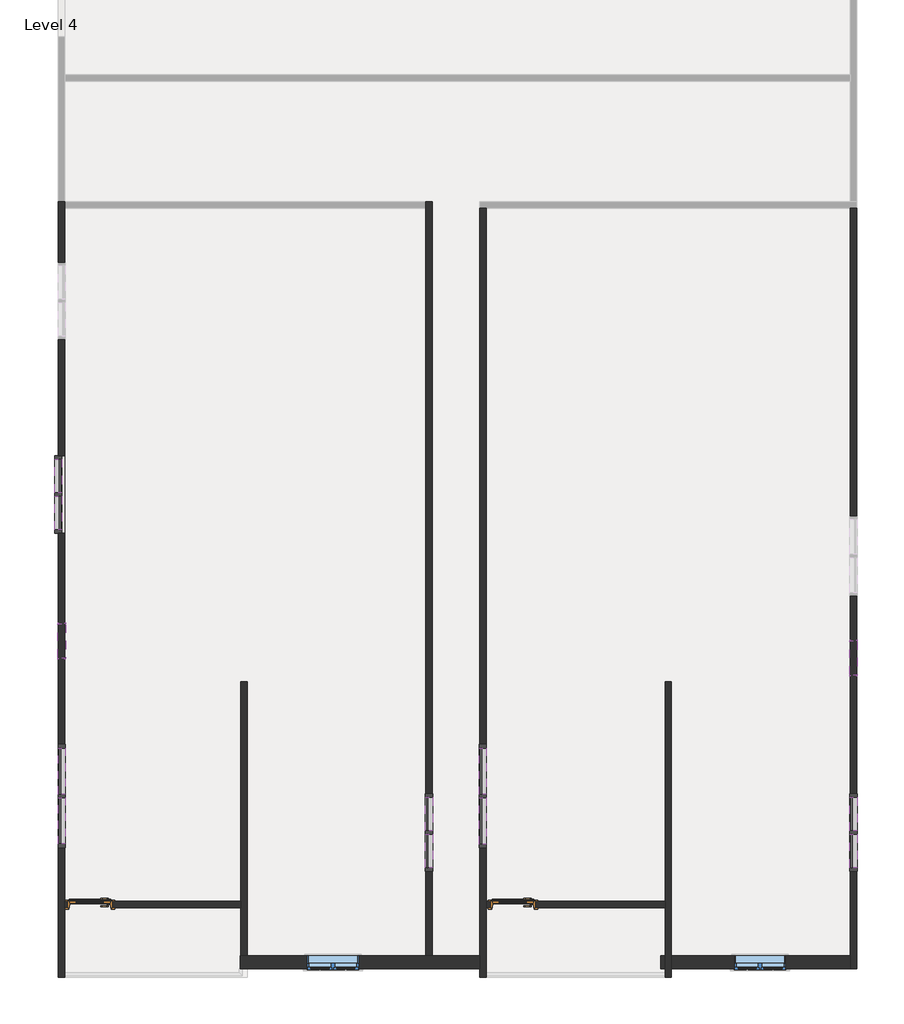
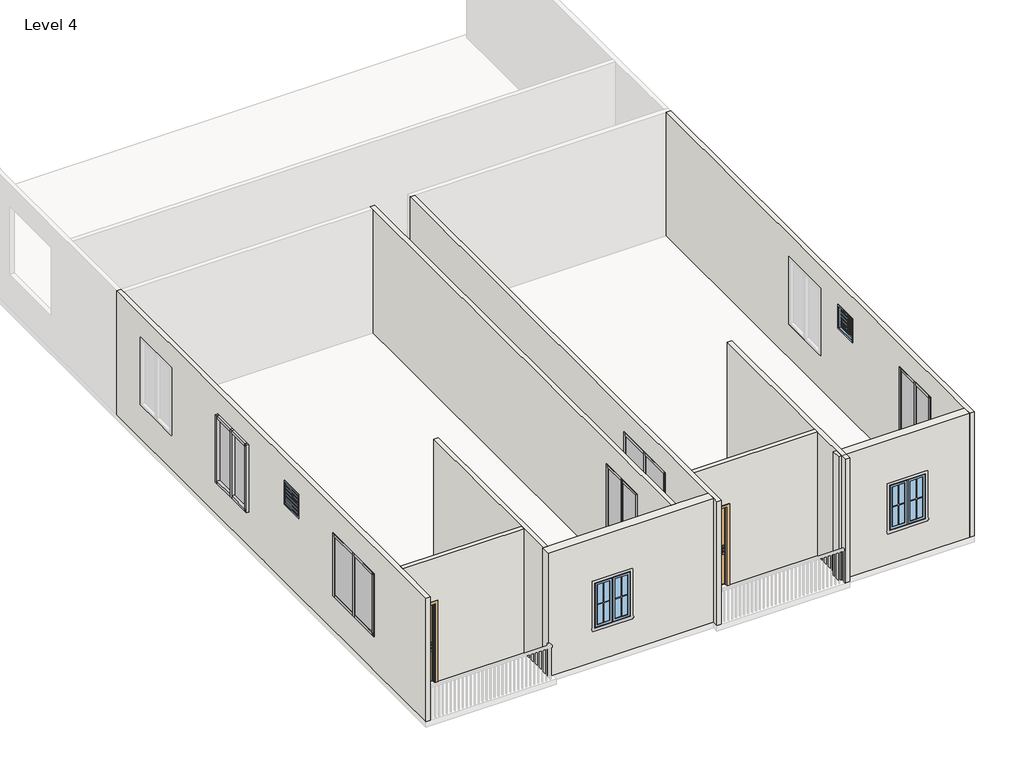
# One storey, part 1 of 3: 35 members, 10 plates, 10 walls, 4 windows, 2 doors.
"""IFC4 building model written with IfcOpenShell, lengths in millimetres."""

from ifc_helpers import new_model, si_unit, frame, origin, place, context, project, spatial, polyline, outline, extrude, faceted_brep, transform, mapped, element, save
from components import door_b81be692, member_8acf8d94, member_501b078b, member_2e6d4a6b, member_96ae0c19, member_d60e8053, member_2fae0574, member_b8ac15de, member_17644e48, system_panel_glazed_c4393626, system_panel_glazed_0e71bc1b, system_panel_glazed_e97abd02, system_panel_glazed_a7ecbca6, window_d341e8ac, window_d39e7ecb

model = new_model("IFC4")

# Units and contexts
model_context = context("Model", 3, world=origin())
ifc_project = project(units=[si_unit("LENGTHUNIT", "METRE", prefix="MILLI")], contexts=[model_context])

# Site, building, storey
site = spatial("IfcSite", under=ifc_project)
building = spatial("IfcBuilding", under=site)
storey = spatial("IfcBuildingStorey", under=building, Name="Level 4", Elevation=10058.4)

# Doors
placement = place(None, origin())
door_shape = door_b81be692(model_context)
element("IfcDoor", 1, ObjectType="29\" x 84\"", at=placement, inside=storey, context=model_context, shape_type="MappedRepresentation", body=[
    mapped(door_shape, transform((-7651.507583, -9448.7163489, 10058.4), x_axis=(1.0, 0.0, 0.0), y_axis=(0.0, 1.0, 0.0), z_axis=(0.0, 0.0, 1.0))),
])
element("IfcDoor", 2, ObjectType="29\" x 84\"", at=placement, inside=storey, context=model_context, shape_type="MappedRepresentation", body=[
    mapped(door_shape, transform((-172.2931282, -9448.9038009, 10058.4), x_axis=(1.0, 0.0, 0.0), y_axis=(0.0, 1.0, 0.0), z_axis=(0.0, 0.0, 1.0))),
])

# Members
member_shape = member_8acf8d94(model_context)
element("IfcMember", 3, ObjectType="Rectangular Mullion : 2.5\" x 5\" rectangular", at=placement, inside=storey, context=model_context, shape_type="MappedRepresentation", body=[
    mapped(member_shape, transform((-8153.157583, -8377.1401329, 12680.286558), x_axis=(0.0, 0.0, 1.0), y_axis=(-1.0, 0.0, 0.0), z_axis=(0.0, -1.0, 0.0))),
])
element("IfcMember", 4, ObjectType="Rectangular Mullion : 2.5\" x 5\" rectangular", at=placement, inside=storey, context=model_context, shape_type="MappedRepresentation", body=[
    mapped(member_shape, transform((-8153.157583, -7497.6651329, 12680.286558), x_axis=(0.0, 0.0, 1.0), y_axis=(-1.0, 0.0, 0.0), z_axis=(0.0, -1.0, 0.0))),
])
element("IfcMember", 5, ObjectType="Rectangular Mullion : 2.5\" x 5\" rectangular", at=placement, inside=storey, context=model_context, shape_type="MappedRepresentation", body=[
    mapped(member_shape, transform((-8153.157583, -6681.6901329, 10972.8), x_axis=(0.0, 0.0, -1.0), y_axis=(-1.0, 0.0, 0.0), z_axis=(0.0, 1.0, 0.0))),
])
element("IfcMember", 6, ObjectType="Rectangular Mullion : 2.5\" x 5\" rectangular", at=placement, inside=storey, context=model_context, shape_type="MappedRepresentation", body=[
    mapped(member_shape, transform((-8153.157583, -7561.1651329, 10972.8), x_axis=(0.0, 0.0, -1.0), y_axis=(-1.0, 0.0, 0.0), z_axis=(0.0, 1.0, 0.0))),
])
member_2_shape = member_501b078b(model_context)
element("IfcMember", 7, ObjectType="Rectangular Mullion : 2.5\" x 5\" rectangular", at=placement, inside=storey, context=model_context, shape_type="MappedRepresentation", body=[
    mapped(member_2_shape, transform((5848.1708786, -8795.0998253, 12801.6), x_axis=(0.0, 0.0, 1.0), y_axis=(-1.0, 0.0, 0.0), z_axis=(0.0, -1.0, 0.0))),
])
element("IfcMember", 8, ObjectType="Rectangular Mullion : 2.5\" x 5\" rectangular", at=placement, inside=storey, context=model_context, shape_type="MappedRepresentation", body=[
    mapped(member_2_shape, transform((5848.1708786, -8142.1745373, 12801.6), x_axis=(0.0, 0.0, 1.0), y_axis=(-1.0, 0.0, 0.0), z_axis=(0.0, -1.0, 0.0))),
])
element("IfcMember", 9, ObjectType="Rectangular Mullion : 2.5\" x 5\" rectangular", at=placement, inside=storey, context=model_context, shape_type="MappedRepresentation", body=[
    mapped(member_2_shape, transform((-1656.4435762, -8795.0998253, 12801.6), x_axis=(0.0, 0.0, 1.0), y_axis=(-1.0, 0.0, 0.0), z_axis=(0.0, -1.0, 0.0))),
])
element("IfcMember", 10, ObjectType="Rectangular Mullion : 2.5\" x 5\" rectangular", at=placement, inside=storey, context=model_context, shape_type="MappedRepresentation", body=[
    mapped(member_2_shape, transform((-1656.4435762, -8142.1745373, 12801.6), x_axis=(0.0, 0.0, 1.0), y_axis=(-1.0, 0.0, 0.0), z_axis=(0.0, -1.0, 0.0))),
])
element("IfcMember", 11, ObjectType="Rectangular Mullion : 2.5\" x 5\" rectangular", at=placement, inside=storey, context=model_context, shape_type="MappedRepresentation", body=[
    mapped(member_2_shape, transform((5848.1708786, -7552.7492493, 10972.8), x_axis=(0.0, 0.0, -1.0), y_axis=(-1.0, 0.0, 0.0), z_axis=(0.0, 1.0, 0.0))),
])
element("IfcMember", 12, ObjectType="Rectangular Mullion : 2.5\" x 5\" rectangular", at=placement, inside=storey, context=model_context, shape_type="MappedRepresentation", body=[
    mapped(member_2_shape, transform((5848.1708786, -8205.6745373, 10972.8), x_axis=(0.0, 0.0, -1.0), y_axis=(-1.0, 0.0, 0.0), z_axis=(0.0, 1.0, 0.0))),
])
element("IfcMember", 13, ObjectType="Rectangular Mullion : 2.5\" x 5\" rectangular", at=placement, inside=storey, context=model_context, shape_type="MappedRepresentation", body=[
    mapped(member_2_shape, transform((-1656.4435762, -7552.7492493, 10972.8), x_axis=(0.0, 0.0, -1.0), y_axis=(-1.0, 0.0, 0.0), z_axis=(0.0, 1.0, 0.0))),
])
element("IfcMember", 14, ObjectType="Rectangular Mullion : 2.5\" x 5\" rectangular", at=placement, inside=storey, context=model_context, shape_type="MappedRepresentation", body=[
    mapped(member_2_shape, transform((-1656.4435762, -8205.6745373, 10972.8), x_axis=(0.0, 0.0, -1.0), y_axis=(-1.0, 0.0, 0.0), z_axis=(0.0, 1.0, 0.0))),
])
member_3_shape = member_2e6d4a6b(model_context)
element("IfcMember", 15, ObjectType="Rectangular Mullion : 2.5\" x 5\" rectangular", at=placement, inside=storey, context=model_context, shape_type="MappedRepresentation", body=[
    mapped(member_3_shape, transform((-705.6931282, -8380.4909009, 12801.6), x_axis=(0.0, 0.0, 1.0), y_axis=(-1.0, 0.0, 0.0), z_axis=(0.0, -1.0, 0.0))),
])
element("IfcMember", 16, ObjectType="Rectangular Mullion : 2.5\" x 5\" rectangular", at=placement, inside=storey, context=model_context, shape_type="MappedRepresentation", body=[
    mapped(member_3_shape, transform((-705.6931282, -7499.3405169, 12801.6), x_axis=(0.0, 0.0, 1.0), y_axis=(-1.0, 0.0, 0.0), z_axis=(0.0, -1.0, 0.0))),
])
element("IfcMember", 17, ObjectType="Rectangular Mullion : 2.5\" x 5\" rectangular", at=placement, inside=storey, context=model_context, shape_type="MappedRepresentation", body=[
    mapped(member_3_shape, transform((-705.6931282, -6681.6901329, 10972.8), x_axis=(0.0, 0.0, -1.0), y_axis=(-1.0, 0.0, 0.0), z_axis=(0.0, 1.0, 0.0))),
])
element("IfcMember", 18, ObjectType="Rectangular Mullion : 2.5\" x 5\" rectangular", at=placement, inside=storey, context=model_context, shape_type="MappedRepresentation", body=[
    mapped(member_3_shape, transform((-705.6931282, -7562.8405169, 10972.8), x_axis=(0.0, 0.0, -1.0), y_axis=(-1.0, 0.0, 0.0), z_axis=(0.0, 1.0, 0.0))),
])
member_4_shape = member_96ae0c19(model_context)
element("IfcMember", 19, ObjectType="Rectangular Mullion : 2.5\" x 5\" rectangular", at=placement, inside=storey, context=model_context, shape_type="MappedRepresentation", body=[
    mapped(member_4_shape, transform((-8210.307583, -2819.4060617, 12801.6), x_axis=(0.0, 0.0, 1.0), y_axis=(-1.0, 0.0, 0.0), z_axis=(0.0, -1.0, 0.0))),
])
element("IfcMember", 20, ObjectType="Rectangular Mullion : 2.5\" x 5\" rectangular", at=placement, inside=storey, context=model_context, shape_type="MappedRepresentation", body=[
    mapped(member_4_shape, transform((-8210.307583, -2164.5788979, 12801.6), x_axis=(0.0, 0.0, 1.0), y_axis=(-1.0, 0.0, 0.0), z_axis=(0.0, -1.0, 0.0))),
])
element("IfcMember", 21, ObjectType="Rectangular Mullion : 2.5\" x 5\" rectangular", at=placement, inside=storey, context=model_context, shape_type="MappedRepresentation", body=[
    mapped(member_4_shape, transform((-8210.307583, -1573.2517341, 10972.8), x_axis=(0.0, 0.0, -1.0), y_axis=(-1.0, 0.0, 0.0), z_axis=(0.0, 1.0, 0.0))),
])
element("IfcMember", 22, ObjectType="Rectangular Mullion : 2.5\" x 5\" rectangular", at=placement, inside=storey, context=model_context, shape_type="MappedRepresentation", body=[
    mapped(member_4_shape, transform((-8210.307583, -2228.0788979, 10972.8), x_axis=(0.0, 0.0, -1.0), y_axis=(-1.0, 0.0, 0.0), z_axis=(0.0, 1.0, 0.0))),
])
member_5_shape = member_d60e8053(model_context)
element("IfcMember", 23, ObjectType="Rectangular Mullion : 2.5\" x 5\" rectangular", at=placement, inside=storey, context=model_context, shape_type="MappedRepresentation", body=[
    mapped(member_5_shape, transform((-8210.307583, -2196.3288979, 10972.8), x_axis=(0.0, -1.0, 0.0), y_axis=(-1.0, 0.0, 0.0), z_axis=(0.0, 0.0, -1.0))),
])
member_6_shape = member_2fae0574(model_context)
element("IfcMember", 24, ObjectType="Rectangular Mullion : 2.5\" x 5\" rectangular", at=placement, inside=storey, context=model_context, shape_type="MappedRepresentation", body=[
    mapped(member_6_shape, transform((-8210.307583, -1509.7517341, 12801.6), x_axis=(0.0, 1.0, 0.0), y_axis=(-1.0, 0.0, 0.0), z_axis=(0.0, 0.0, 1.0))),
])
element("IfcMember", 25, ObjectType="Rectangular Mullion : 2.5\" x 5\" rectangular", at=placement, inside=storey, context=model_context, shape_type="MappedRepresentation", body=[
    mapped(member_6_shape, transform((-8210.307583, -2882.9060617, 10972.8), x_axis=(0.0, -1.0, 0.0), y_axis=(-1.0, 0.0, 0.0), z_axis=(0.0, 0.0, -1.0))),
])
member_7_shape = member_b8ac15de(model_context)
element("IfcMember", 26, ObjectType="Rectangular Mullion : 2.5\" x 5\" rectangular", at=placement, inside=storey, context=model_context, shape_type="MappedRepresentation", body=[
    mapped(member_7_shape, transform((-8153.157583, -7529.4151329, 10972.8), x_axis=(0.0, -1.0, 0.0), y_axis=(-1.0, 0.0, 0.0), z_axis=(0.0, 0.0, -1.0))),
])
member_8_shape = member_17644e48(model_context)
element("IfcMember", 27, ObjectType="Rectangular Mullion : 2.5\" x 5\" rectangular", at=placement, inside=storey, context=model_context, shape_type="MappedRepresentation", body=[
    mapped(member_8_shape, transform((-8153.157583, -6618.1901329, 12680.286558), x_axis=(0.0, 1.0, 0.0), y_axis=(-1.0, 0.0, 0.0), z_axis=(0.0, 0.0, 1.0))),
])
element("IfcMember", 28, ObjectType="Rectangular Mullion : 2.5\" x 5\" rectangular", at=placement, inside=storey, context=model_context, shape_type="MappedRepresentation", body=[
    mapped(member_8_shape, transform((-8153.157583, -8440.6401329, 10972.8), x_axis=(0.0, -1.0, 0.0), y_axis=(-1.0, 0.0, 0.0), z_axis=(0.0, 0.0, -1.0))),
])
element("IfcMember", 29, ObjectType="Rectangular Mullion : 2.5\" x 5\" rectangular", at=placement, inside=storey, context=model_context, shape_type="MappedRepresentation", body=[
    mapped(member_5_shape, transform((5848.1708786, -8173.9245373, 10972.8), x_axis=(0.0, -1.0, 0.0), y_axis=(-1.0, 0.0, 0.0), z_axis=(0.0, 0.0, -1.0))),
])
element("IfcMember", 30, ObjectType="Rectangular Mullion : 2.5\" x 5\" rectangular", at=placement, inside=storey, context=model_context, shape_type="MappedRepresentation", body=[
    mapped(member_5_shape, transform((-1656.4435762, -8173.9245373, 10972.8), x_axis=(0.0, -1.0, 0.0), y_axis=(-1.0, 0.0, 0.0), z_axis=(0.0, 0.0, -1.0))),
])
element("IfcMember", 31, ObjectType="Rectangular Mullion : 2.5\" x 5\" rectangular", at=placement, inside=storey, context=model_context, shape_type="MappedRepresentation", body=[
    mapped(member_5_shape, transform((-705.6931282, -7531.0905169, 10972.8), x_axis=(0.0, -1.0, 0.0), y_axis=(-1.0, 0.0, 0.0), z_axis=(0.0, 0.0, -1.0))),
])
element("IfcMember", 32, ObjectType="Rectangular Mullion : 2.5\" x 5\" rectangular", at=placement, inside=storey, context=model_context, shape_type="MappedRepresentation", body=[
    mapped(member_6_shape, transform((5848.1708786, -7489.2492493, 12801.6), x_axis=(0.0, 1.0, 0.0), y_axis=(-1.0, 0.0, 0.0), z_axis=(0.0, 0.0, 1.0))),
])
element("IfcMember", 33, ObjectType="Rectangular Mullion : 2.5\" x 5\" rectangular", at=placement, inside=storey, context=model_context, shape_type="MappedRepresentation", body=[
    mapped(member_6_shape, transform((-1656.4435762, -7489.2492493, 12801.6), x_axis=(0.0, 1.0, 0.0), y_axis=(-1.0, 0.0, 0.0), z_axis=(0.0, 0.0, 1.0))),
])
element("IfcMember", 34, ObjectType="Rectangular Mullion : 2.5\" x 5\" rectangular", at=placement, inside=storey, context=model_context, shape_type="MappedRepresentation", body=[
    mapped(member_6_shape, transform((-705.6931282, -6618.1901329, 12801.6), x_axis=(0.0, 1.0, 0.0), y_axis=(-1.0, 0.0, 0.0), z_axis=(0.0, 0.0, 1.0))),
])
element("IfcMember", 35, ObjectType="Rectangular Mullion : 2.5\" x 5\" rectangular", at=placement, inside=storey, context=model_context, shape_type="MappedRepresentation", body=[
    mapped(member_6_shape, transform((5848.1708786, -8858.5998253, 10972.8), x_axis=(0.0, -1.0, 0.0), y_axis=(-1.0, 0.0, 0.0), z_axis=(0.0, 0.0, -1.0))),
])
element("IfcMember", 36, ObjectType="Rectangular Mullion : 2.5\" x 5\" rectangular", at=placement, inside=storey, context=model_context, shape_type="MappedRepresentation", body=[
    mapped(member_6_shape, transform((-1656.4435762, -8858.5998253, 10972.8), x_axis=(0.0, -1.0, 0.0), y_axis=(-1.0, 0.0, 0.0), z_axis=(0.0, 0.0, -1.0))),
])
element("IfcMember", 37, ObjectType="Rectangular Mullion : 2.5\" x 5\" rectangular", at=placement, inside=storey, context=model_context, shape_type="MappedRepresentation", body=[
    mapped(member_6_shape, transform((-705.6931282, -8443.9909009, 10972.8), x_axis=(0.0, -1.0, 0.0), y_axis=(-1.0, 0.0, 0.0), z_axis=(0.0, 0.0, -1.0))),
])

# Plates
system_panel_glazed_shape = system_panel_glazed_c4393626(model_context)
element("IfcPlate", 38, ObjectType="System Panel : Glazed", at=placement, inside=storey, context=model_context, shape_type="MappedRepresentation", body=[
    mapped(system_panel_glazed_shape, transform((-8210.307583, -1868.915316, 11036.3), x_axis=(0.0, -1.0, 0.0), y_axis=(1.0, 0.0, 0.0), z_axis=(0.0, 0.0, 1.0))),
])
element("IfcPlate", 39, ObjectType="System Panel : Glazed", at=placement, inside=storey, context=model_context, shape_type="MappedRepresentation", body=[
    mapped(system_panel_glazed_shape, transform((-8210.307583, -2523.7424798, 11036.3), x_axis=(0.0, -1.0, 0.0), y_axis=(1.0, 0.0, 0.0), z_axis=(0.0, 0.0, 1.0))),
])
system_panel_glazed_2_shape = system_panel_glazed_0e71bc1b(model_context)
element("IfcPlate", 40, ObjectType="System Panel : Glazed", at=placement, inside=storey, context=model_context, shape_type="MappedRepresentation", body=[
    mapped(system_panel_glazed_2_shape, transform((-8153.157583, -7089.6776329, 11036.3), x_axis=(0.0, -1.0, 0.0), y_axis=(1.0, 0.0, 0.0), z_axis=(0.0, 0.0, 1.0))),
])
element("IfcPlate", 41, ObjectType="System Panel : Glazed", at=placement, inside=storey, context=model_context, shape_type="MappedRepresentation", body=[
    mapped(system_panel_glazed_2_shape, transform((-8153.157583, -7969.1526329, 11036.3), x_axis=(0.0, -1.0, 0.0), y_axis=(1.0, 0.0, 0.0), z_axis=(0.0, 0.0, 1.0))),
])
system_panel_glazed_3_shape = system_panel_glazed_e97abd02(model_context)
element("IfcPlate", 42, ObjectType="System Panel : Glazed", at=placement, inside=storey, context=model_context, shape_type="MappedRepresentation", body=[
    mapped(system_panel_glazed_3_shape, transform((5848.1708786, -7847.4618933, 11036.3), x_axis=(0.0, -1.0, 0.0), y_axis=(1.0, 0.0, 0.0), z_axis=(0.0, 0.0, 1.0))),
])
element("IfcPlate", 43, ObjectType="System Panel : Glazed", at=placement, inside=storey, context=model_context, shape_type="MappedRepresentation", body=[
    mapped(system_panel_glazed_3_shape, transform((-1656.4435762, -7847.4618933, 11036.3), x_axis=(0.0, -1.0, 0.0), y_axis=(1.0, 0.0, 0.0), z_axis=(0.0, 0.0, 1.0))),
])
element("IfcPlate", 44, ObjectType="System Panel : Glazed", at=placement, inside=storey, context=model_context, shape_type="MappedRepresentation", body=[
    mapped(system_panel_glazed_3_shape, transform((5848.1708786, -8500.3871813, 11036.3), x_axis=(0.0, -1.0, 0.0), y_axis=(1.0, 0.0, 0.0), z_axis=(0.0, 0.0, 1.0))),
])
element("IfcPlate", 45, ObjectType="System Panel : Glazed", at=placement, inside=storey, context=model_context, shape_type="MappedRepresentation", body=[
    mapped(system_panel_glazed_3_shape, transform((-1656.4435762, -8500.3871813, 11036.3), x_axis=(0.0, -1.0, 0.0), y_axis=(1.0, 0.0, 0.0), z_axis=(0.0, 0.0, 1.0))),
])
system_panel_glazed_4_shape = system_panel_glazed_a7ecbca6(model_context)
element("IfcPlate", 46, ObjectType="System Panel : Glazed", at=placement, inside=storey, context=model_context, shape_type="MappedRepresentation", body=[
    mapped(system_panel_glazed_4_shape, transform((-705.6931282, -7090.5153249, 11036.3), x_axis=(0.0, -1.0, 0.0), y_axis=(1.0, 0.0, 0.0), z_axis=(0.0, 0.0, 1.0))),
])
element("IfcPlate", 47, ObjectType="System Panel : Glazed", at=placement, inside=storey, context=model_context, shape_type="MappedRepresentation", body=[
    mapped(system_panel_glazed_4_shape, transform((-705.6931282, -7971.6657089, 11036.3), x_axis=(0.0, -1.0, 0.0), y_axis=(1.0, 0.0, 0.0), z_axis=(0.0, 0.0, 1.0))),
])

# Walls
element("IfcWall", 48, ObjectType="4.5\" wall", at=placement, inside=storey, context=model_context, shape_type="Brep", body=[
    faceted_brep([(-8096.007583, -10738.0280197, 10058.4), (-8096.007583, -9509.0413489, 10058.4), (-8096.007583, -9394.7413489, 10058.4), (-8096.007583, 2864.0002499, 10058.4), (-8096.007583, 2978.3002499, 10058.4), (-8096.007583, 2978.3002499, 13411.2), (-8096.007583, 2864.0002499, 13411.2), (-8096.007583, -9394.7413489, 13411.2), (-8096.007583, -9509.0413489, 13411.2), (-8096.007583, -10738.0280197, 13411.2), (-8096.007583, -6618.1901329, 12680.286558), (-8096.007583, -6618.1901329, 10972.8), (-8096.007583, -8440.6401329, 10972.8), (-8096.007583, -8440.6401329, 12680.286558), (-8096.007583, -5094.1901329, 12172.95), (-8096.007583, -5094.1901329, 12782.55), (-8096.007583, -4484.5901329, 12782.55), (-8096.007583, -4484.5901329, 12172.95), (-8096.007583, 1909.8209543, 12801.6), (-8096.007583, 1909.8209543, 10972.8), (-8096.007583, 536.6666267, 10972.8), (-8096.007583, 536.6666267, 12801.6), (-8096.007583, -1509.7517341, 12801.6), (-8096.007583, -1509.7517341, 10972.8), (-8096.007583, -2882.9060617, 10972.8), (-8096.007583, -2882.9060617, 12801.6), (-8210.307583, 2978.3002499, 10058.4), (-8210.307583, -10738.0280197, 10058.4), (-8210.307583, -10738.0280197, 13411.2), (-8210.307583, 2978.3002499, 13411.2), (-8210.307583, -6618.1901329, 10972.8), (-8210.307583, -6618.1901329, 12680.286558), (-8210.307583, -8440.6401329, 12680.286558), (-8210.307583, -8440.6401329, 10972.8), (-8210.307583, -5094.1901329, 12782.55), (-8210.307583, -5094.1901329, 12172.95), (-8210.307583, -4484.5901329, 12172.95), (-8210.307583, -4484.5901329, 12782.55), (-8210.307583, 1909.8209543, 10972.8), (-8210.307583, 1909.8209543, 12801.6), (-8210.307583, 536.6666267, 12801.6), (-8210.307583, 536.6666267, 10972.8), (-8210.307583, -1509.7517341, 10972.8), (-8210.307583, -1509.7517341, 12801.6), (-8210.307583, -2882.9060617, 12801.6), (-8210.307583, -2882.9060617, 10972.8)], [[[0, 1, 2, 3, 4, 5, 6, 7, 8, 9], [10, 11, 12, 13], [14, 15, 16, 17], [18, 19, 20, 21], [22, 23, 24, 25]], [[26, 27, 28, 29], [30, 31, 32, 33], [34, 35, 36, 37], [38, 39, 40, 41], [42, 43, 44, 45]], [[4, 3, 2, 1, 0, 27, 26]], [[9, 8, 7, 6, 5, 29, 28]], [[0, 9, 28, 27]], [[5, 4, 26, 29]], [[10, 31, 30, 11]], [[31, 10, 13, 32]], [[32, 13, 12, 33]], [[11, 30, 33, 12]], [[35, 34, 15, 14]], [[36, 35, 14, 17]], [[37, 36, 17, 16]], [[34, 37, 16, 15]], [[38, 19, 18, 39]], [[39, 18, 21, 40]], [[40, 21, 20, 41]], [[19, 38, 41, 20]], [[22, 43, 42, 23]], [[43, 22, 25, 44]], [[44, 25, 24, 45]], [[23, 42, 45, 24]]]),
])
element("IfcWall", 49, ObjectType="4.5\" wall", at=placement, inside=storey, context=model_context, shape_type="Brep", body=[
    faceted_brep([(-1599.2935762, -10357.2779557, 10058.4), (-1599.2935762, 2978.3002499, 10058.4), (-1599.2935762, 2978.3002499, 13411.2), (-1599.2935762, -10357.2779557, 13411.2), (-1599.2935762, -7489.2492493, 12801.6), (-1599.2935762, -7489.2492493, 10972.8), (-1599.2935762, -8858.5998253, 10972.8), (-1599.2935762, -8858.5998253, 12801.6), (-1713.5935762, 2978.3002499, 10058.4), (-1713.5935762, 2864.0002499, 10058.4), (-1713.5935762, -10357.2779557, 10058.4), (-1713.5935762, -10357.2779557, 13411.2), (-1713.5935762, 2864.0002499, 13411.2), (-1713.5935762, 2978.3002499, 13411.2), (-1713.5935762, -7489.2492493, 10972.8), (-1713.5935762, -7489.2492493, 12801.6), (-1713.5935762, -8858.5998253, 12801.6), (-1713.5935762, -8858.5998253, 10972.8)], [[[0, 1, 2, 3], [4, 5, 6, 7]], [[8, 9, 10, 11, 12, 13], [14, 15, 16, 17]], [[1, 0, 10, 9, 8]], [[3, 2, 13, 12, 11]], [[2, 1, 8, 13]], [[0, 3, 11, 10]], [[14, 5, 4, 15]], [[15, 4, 7, 16]], [[16, 7, 6, 17]], [[5, 14, 17, 6]]]),
])
element("IfcWall", 50, ObjectType="4.5\" wall", at=placement, inside=storey, context=model_context, shape_type="Brep", body=[
    faceted_brep([(5791.0208786, 2864.0002499, 10058.4), (5791.0208786, -10357.2779557, 10058.4), (5791.0208786, -10585.8779557, 10058.4), (5791.0208786, -10585.8779557, 13411.2), (5791.0208786, -10357.2779557, 13411.2), (5791.0208786, 2864.0002499, 13411.2), (5791.0208786, -7489.2492493, 10972.8), (5791.0208786, -7489.2492493, 12801.6), (5791.0208786, -8858.5998253, 12801.6), (5791.0208786, -8858.5998253, 10972.8), (5791.0208786, -2574.8021821, 10972.8), (5791.0208786, -2574.8021821, 12801.6), (5791.0208786, -3997.2021821, 12801.6), (5791.0208786, -3997.2021821, 10972.8), (5791.0208786, -4784.6021821, 12211.05), (5791.0208786, -4784.6021821, 12820.65), (5791.0208786, -5394.2021821, 12820.65), (5791.0208786, -5394.2021821, 12211.05), (5905.3208786, -10585.8779557, 10058.4), (5905.3208786, 2864.0002499, 10058.4), (5905.3208786, 2864.0002499, 13411.2), (5905.3208786, -10585.8779557, 13411.2), (5905.3208786, -7489.2492493, 12801.6), (5905.3208786, -7489.2492493, 10972.8), (5905.3208786, -8858.5998253, 10972.8), (5905.3208786, -8858.5998253, 12801.6), (5905.3208786, -2574.8021821, 12801.6), (5905.3208786, -2574.8021821, 10972.8), (5905.3208786, -3997.2021821, 10972.8), (5905.3208786, -3997.2021821, 12801.6), (5905.3208786, -4784.6021821, 12820.65), (5905.3208786, -4784.6021821, 12211.05), (5905.3208786, -5394.2021821, 12211.05), (5905.3208786, -5394.2021821, 12820.65)], [[[0, 1, 2, 3, 4, 5], [6, 7, 8, 9], [10, 11, 12, 13], [14, 15, 16, 17]], [[18, 19, 20, 21], [22, 23, 24, 25], [26, 27, 28, 29], [30, 31, 32, 33]], [[2, 1, 0, 19, 18]], [[5, 4, 3, 21, 20]], [[0, 5, 20, 19]], [[3, 2, 18, 21]], [[22, 7, 6, 23]], [[7, 22, 25, 8]], [[8, 25, 24, 9]], [[23, 6, 9, 24]], [[10, 27, 26, 11]], [[11, 26, 29, 12]], [[12, 29, 28, 13]], [[27, 10, 13, 28]], [[31, 30, 15, 14]], [[32, 31, 14, 17]], [[33, 32, 17, 16]], [[30, 33, 16, 15]]]),
])
element("IfcWall", 51, ObjectType="4.5\" wall", at=placement, inside=storey, context=model_context, shape_type="Brep", body=[
    faceted_brep([(-762.8431282, 2864.0002499, 10058.4), (-762.8431282, -10357.2779557, 10058.4), (-762.8431282, -10585.8779557, 10058.4), (-762.8431282, -10737.6531157, 10058.4), (-762.8431282, -10737.6531157, 13411.2), (-762.8431282, -10585.8779557, 13411.2), (-762.8431282, -10357.2779557, 13411.2), (-762.8431282, 2864.0002499, 13411.2), (-762.8431282, -6618.1901329, 10972.8), (-762.8431282, -6618.1901329, 12801.6), (-762.8431282, -8443.9909009, 12801.6), (-762.8431282, -8443.9909009, 10972.8), (-648.5431282, -10737.6531157, 10058.4), (-648.5431282, -9509.2288009, 10058.4), (-648.5431282, -9394.9288009, 10058.4), (-648.5431282, 2864.0002499, 10058.4), (-648.5431282, 2864.0002499, 13411.2), (-648.5431282, -9394.9288009, 13411.2), (-648.5431282, -9509.2288009, 13411.2), (-648.5431282, -10737.6531157, 13411.2), (-648.5431282, -6618.1901329, 12801.6), (-648.5431282, -6618.1901329, 10972.8), (-648.5431282, -8443.9909009, 10972.8), (-648.5431282, -8443.9909009, 12801.6)], [[[0, 1, 2, 3, 4, 5, 6, 7], [8, 9, 10, 11]], [[12, 13, 14, 15, 16, 17, 18, 19], [20, 21, 22, 23]], [[3, 2, 1, 0, 15, 14, 13, 12]], [[4, 3, 12, 19]], [[7, 6, 5, 4, 19, 18, 17, 16]], [[8, 21, 20, 9]], [[9, 20, 23, 10]], [[10, 23, 22, 11]], [[21, 8, 11, 22]], [[0, 7, 16, 15]]]),
])
element("IfcWall", 52, ObjectType="4.5\" wall", at=placement, inside=storey, context=model_context, shape_type="Brep", body=[
    faceted_brep([(-4874.3237038, -10357.2779557, 10058.4), (-4874.3237038, -5507.4946657, 10058.4), (-4874.3237038, -5507.4946657, 13411.2), (-4874.3237038, -10357.2779557, 13411.2), (-4988.6237038, -10357.2779557, 10058.4), (-4988.6237038, -10357.2779557, 13411.2), (-4988.6237038, -9509.0413489, 13411.2), (-4988.6237038, -9394.7413489, 13411.2), (-4988.6237038, -5507.4946657, 13411.2), (-4988.6237038, -5507.4946657, 10058.4), (-4988.6237038, -9394.7413489, 10058.4), (-4988.6237038, -9509.0413489, 10058.4)], [[[0, 1, 2, 3]], [[4, 5, 6, 7, 8, 9, 10, 11]], [[1, 0, 4, 11, 10, 9]], [[2, 1, 9, 8]], [[3, 2, 8, 7, 6, 5]], [[0, 3, 5, 4]]]),
])
element("IfcWall", 53, ObjectType="4.5\" wall", at=placement, inside=storey, context=model_context, shape_type="Brep", body=[
    faceted_brep([(2515.990751, -5507.4946657, 10058.4), (2515.990751, -9394.9288009, 10058.4), (2515.990751, -9509.2288009, 10058.4), (2515.990751, -10737.6531157, 10058.4), (2515.990751, -10737.6531157, 13411.2), (2515.990751, -9509.2288009, 13411.2), (2515.990751, -9394.9288009, 13411.2), (2515.990751, -5507.4946657, 13411.2), (2630.290751, -5507.4946657, 10058.4), (2630.290751, -5507.4946657, 13411.2), (2630.290751, -10737.6531157, 13411.2), (2630.290751, -10737.6531157, 10058.4)], [[[0, 1, 2, 3, 4, 5, 6, 7]], [[8, 9, 10, 11]], [[3, 2, 1, 0, 8, 11]], [[4, 3, 11, 10]], [[7, 6, 5, 4, 10, 9]], [[0, 7, 9, 8]]]),
])
element("IfcWall", 54, ObjectType="4.5\" wall", at=placement, inside=storey, context=model_context, shape_type="SweptSolid", body=[
    extrude(outline(polyline([(13411.2, -4988.6237038), (13411.2, -8096.007583), (10058.4, -8096.007583), (10058.4, -8045.207583), (12217.4, -8045.207583), (12217.4, -7257.807583), (10058.4, -7257.807583), (10058.4, -4988.6237038), (13411.2, -4988.6237038)])), frame((0.0, -9509.0413489, 0.0), z_axis=(0.0, 1.0, 0.0), x_axis=(0.0, 0.0, 1.0)), (0.0, 0.0, 1.0), 114.3),
])
element("IfcWall", 55, ObjectType="4.5\" wall", at=placement, inside=storey, context=model_context, shape_type="SweptSolid", body=[
    extrude(outline(polyline([(13411.2, 2515.990751), (13411.2, -648.5431282), (10058.4, -648.5431282), (10058.4, -565.9931282), (12217.4, -565.9931282), (12217.4, 221.4068718), (10058.4, 221.4068718), (10058.4, 2515.990751), (13411.2, 2515.990751)])), frame((0.0, -9509.2288009, 0.0), z_axis=(0.0, 1.0, 0.0), x_axis=(0.0, 0.0, 1.0)), (0.0, 0.0, 1.0), 114.3),
])
element("IfcWall", 56, ObjectType="9\" wall", at=placement, inside=storey, context=model_context, shape_type="Brep", body=[
    faceted_brep([(-762.8431282, -10357.2779557, 10058.4), (-1599.2935762, -10357.2779557, 10058.4), (-1713.5935762, -10357.2779557, 10058.4), (-4874.3237038, -10357.2779557, 10058.4), (-4988.6237038, -10357.2779557, 10058.4), (-4996.231207, -10357.2779557, 10058.4), (-4996.231207, -10357.2779557, 13411.2), (-4988.6237038, -10357.2779557, 13411.2), (-4874.3237038, -10357.2779557, 13411.2), (-1713.5935762, -10357.2779557, 13411.2), (-1599.2935762, -10357.2779557, 13411.2), (-762.8431282, -10357.2779557, 13411.2), (-3813.8737038, -10357.2779557, 12192.0), (-3813.8737038, -10357.2779557, 10972.8), (-2899.4737038, -10357.2779557, 10972.8), (-2899.4737038, -10357.2779557, 12192.0), (-762.8431282, -10585.8779557, 10058.4), (-762.8431282, -10585.8779557, 13411.2), (-4996.231207, -10585.8779557, 13411.2), (-4996.231207, -10585.8779557, 10058.4), (-3813.8737038, -10585.8779557, 12192.0), (-2899.4737038, -10585.8779557, 12192.0), (-2899.4737038, -10585.8779557, 10972.8), (-3813.8737038, -10585.8779557, 10972.8)], [[[0, 1, 2, 3, 4, 5, 6, 7, 8, 9, 10, 11], [12, 13, 14, 15]], [[16, 17, 18, 19], [20, 21, 22, 23]], [[5, 4, 3, 2, 1, 0, 16, 19]], [[6, 5, 19, 18]], [[11, 10, 9, 8, 7, 6, 18, 17]], [[0, 11, 17, 16]], [[13, 12, 20, 23]], [[14, 13, 23, 22]], [[15, 14, 22, 21]], [[12, 15, 21, 20]]]),
])
element("IfcWall", 57, ObjectType="9\" wall", at=placement, inside=storey, context=model_context, shape_type="SweptSolid", body=[
    extrude(outline(polyline([(10058.4, 5791.0208786), (13411.2, 5791.0208786), (13411.2, 2436.2994194), (10058.4, 2436.2994194), (10058.4, 5791.0208786)]), holes=[polyline([(12192.0, 3739.9708786), (12192.0, 4654.3708786), (10972.8, 4654.3708786), (10972.8, 3739.9708786), (12192.0, 3739.9708786)])]), frame((0.0, -10585.8779557, 0.0), z_axis=(0.0, 1.0, 0.0), x_axis=(0.0, 0.0, 1.0)), (0.0, 0.0, 1.0), 228.6),
])

# Windows
window_shape = window_d341e8ac(model_context)
element("IfcWindow", 58, ObjectType="Window-Casement-Double : 36\" x 48\"", at=placement, inside=storey, context=model_context, shape_type="MappedRepresentation", body=[
    mapped(window_shape, transform((-3356.6737038, -10471.5779557, 10058.4), x_axis=(-1.0, 0.0, 0.0), y_axis=(0.0, -1.0, 0.0), z_axis=(0.0, 0.0, 1.0))),
])
element("IfcWindow", 59, ObjectType="Window-Casement-Double : 36\" x 48\"", at=placement, inside=storey, context=model_context, shape_type="MappedRepresentation", body=[
    mapped(window_shape, transform((4197.1708786, -10471.5779557, 10058.4), x_axis=(-1.0, 0.0, 0.0), y_axis=(0.0, -1.0, 0.0), z_axis=(0.0, 0.0, 1.0))),
])
window_2_shape = window_d39e7ecb(model_context)
element("IfcWindow", 60, ObjectType="Window-Louvers : 24\" x 24\"", at=placement, inside=storey, context=model_context, shape_type="MappedRepresentation", body=[
    mapped(window_2_shape, transform((-8159.507583, -4789.3901329, 11258.55), x_axis=(0.0, 1.0, 0.0), y_axis=(-1.0, 0.0, 0.0), z_axis=(0.0, 0.0, 1.0))),
])
element("IfcWindow", 61, ObjectType="Window-Louvers : 24\" x 24\"", at=placement, inside=storey, context=model_context, shape_type="MappedRepresentation", body=[
    mapped(window_2_shape, transform((5854.5208786, -5089.4021821, 11296.65), x_axis=(0.0, -1.0, 0.0), y_axis=(1.0, 0.0, 0.0), z_axis=(0.0, 0.0, 1.0))),
])

save(model, "model.ifc")

# Revit data of these elements
# Type "29\" x 84\""
#   Type Mark = "8"
#   Assembly Code = "B2030100"
#   Analytic Construction = "French door, wood frame with single glass"
#   Threshold Offset [instance default] = 0' - 0 1/2"
#   Thickness = 0' - 1 3/8"
#   Thermal Resistance (R) = 1.0696 (h·ft²·°F)/BTU
#   Swing Angle [instance default] = 90.00°
#   Stiles = 0' - 4 3/4"
#   Rough Width = 2' - 7"
#   Rough Height = 7' - 1"
#   Radius = 1' - 0.00625"
#   Lock Rail = 0' - 7 1/8"
#   Height = 7' - 0"
#   Width = 2' - 5"
#   Heat Transfer Coefficient (U) = 0.9350 BTU/(h·ft²·°F)
#   Door Offset [instance default] = 0' - 0"
#   Bottom Rail = 0' - 9 1/2"
#   Threshold [instance default] = yes
#   Function = 1
#   Exterior Trim [instance default] = yes
#   Trim Material = Cherry
#   Threshold Material = Cherry
#   Panel Material = Cherry
#   Glazing = Glass
#   Frame Material = Cherry
#   Door Handle Material = Aluminum
#   Visual Light Transmittance = 0
#   Solar Heat Gain Coefficient = 0
#   Wall Closure = (empty or 0)
#   Construction Type = (empty or 0)
# Type "Rectangular Mullion : 2.5\" x 5\" rectangular"
#   built-in parameter 1007304 = 0.416667 (stored number, unit not read)
#   built-in parameter 1007301 = 0.104167 (stored number, unit not read)
#   built-in parameter 1007300 = 0.104167 (stored number, unit not read)
# Type "System Panel : Glazed"
#   Construction Type Id = "GSP4R"
#   Analytic Construction = "1/8 in Pilkington single glazing"
#   Visual Light Transmittance = 0.9
#   Solar Heat Gain Coefficient = 0.86
#   Heat Transfer Coefficient (U) = 1.18115 BTU/(h·ft²·°F)
#   Define Thermal Properties by = 1
# Type "4.5\" wall"
#   Assembly Code = "B2010"
#   Layers, outside or top first: 0' - 4 1/2" no material (function 1)
# Type "9\" wall"
#   Assembly Code = "B2010"
#   Layers, outside or top first: 0' - 9" no material (function 1)
# Type "Window-Casement-Double : 36\" x 48\""
#   Type Mark = "14"
#   Fire Rating = "0.5h"
#   Assembly Code = "B2020100"
#   Analytic Construction = "Double glazing - domestic"
#   Frame Extension [instance default] = 0' - 0 1/4"
#   Window Inset [instance default] = 0' - 0"
#   Wall Thickness [instance default] = 0' - 6"
#   Interior Wall Closure [instance default] = 0' - 2 1/4"
#   Half Width = 1' - 6"
#   Visual Light Transmittance = 0.81
#   Thermal Resistance (R) = 1.8146 (h·ft²·°F)/BTU
#   Solar Heat Gain Coefficient = 0.76
#   Rough Width = 3' - 0 1/2"
#   Rough Height = 4' - 0 1/2"
#   Height = 4' - 0"
#   Heat Transfer Coefficient (U) = 0.5511 BTU/(h·ft²·°F)
#   Exterior Wall Closure [instance default] = 0' - 1 1/4"
#   Extension Jamb [instance default] = 0' - 2 1/4"
#   Default Sill Height = 3' - 0"
#   Width = 3' - 0"
#   Define Thermal Properties by = 0
#   Muntin Visibility = yes
#   Interior Trim Visibility [instance default] = yes
#   Exterior Trim Visibility [instance default] = yes
#   Extension Jamb Visibility [instance default] = yes
#   Interior Trim Material = Wood - Stained
#   Muntin Pattern = Muntin Pattern_2x2 : Muntin Pattern_2x2
#   Interior Trim = Trim-Window-Interior-Flat : Picture Frame
#   Interior Frame Material = Wood - Stained
#   Glass Panel Material = Glass
#   Exterior Trim Material = Clad - White
#   Exterior Trim = Trim-Window-Exterior-Flat : with Sill
#   Exterior Frame Material = Clad - White
#   Wall Closure = (empty or 0)
# Type "Window-Louvers : 24\" x 24\""
#   Type Mark = "18"
#   Construction Type Id = "GSP4R"
#   Assembly Code = "B20"
#   Analytic Construction = "1/8 in Pilkington single glazing"
#   Visual Light Transmittance = 0.9
#   Thermal Resistance (R) = 1.53941 (h·ft²·°F)/BTU
#   Solar Heat Gain Coefficient = 0.78
#   Max Height = 1' - 11.74264"
#   Height = 2' - 0"
#   Heat Transfer Coefficient (U) = 0.6496 BTU/(h·ft²·°F)
#   Blade Width [instance default] = 1' - 10 1/2"
#   Blade Vertical Thickness = 0' - 0.35355"
#   Blade Thickness = 0' - 0 1/4"
#   Blade Spacing = 0' - 1 1/2"
#   Blade Height = 0' - 1.85355"
#   Blade Depth = 0' - 3"
#   Blade Angle = 45.00°
#   Default Sill Height = 3' - 0"
#   Trim Projection_Exterior = 0' - 0 1/2"
#   Trim Projection_Interior = 0' - 0 1/2"
#   Trim Width_Exterior = 0' - 1 1/2"
#   Trim Width_Interior = 0' - 1 1/2"
#   Width = 2' - 0"
#   Max Blade Count = 12
#   Define Thermal Properties by = 1
#   Blade Count = 12
#   Frame Material = Birch
#   Louver Material = Birch
#   Trim Exterior Material = Birch
#   Trim Interior Material = Birch
#   Wall Closure = (empty or 0)
# Elements 1, 2 (IfcDoor, "29\" x 84\"")
#   Threshold Offset = 0' - 0 1/2"
#   Swing Angle = 90.00°
#   Door Offset = 0' - 0"
#   Threshold = yes
#   Exterior Trim = yes
#   Phase Created = New Construction
#   Materials on its faces: "Cherry", "Aluminum", "Glass"
# Elements 3, 4, 5, 6, 7, 8, 9, 10, 11, 12, 13, 14, 15, 16, 17, 18, 19, 20, 21, 22, 23, 24, 25, 26, 27, 28, 29, 30, 31, 32, 33, 34, 35, 36, 37 (IfcMember, "Rectangular Mullion : 2.5\" x 5\" rectangular")
#   Phase Created = New Construction
#   Materials on its faces: "Aluminum"
# Elements 38, 39, 40, 41, 42, 43, 44, 45, 46, 47 (IfcPlate, "System Panel : Glazed")
#   Phase Created = New Construction
#   Materials on its faces: "Glass"
# Elements 48, 49, 50, 51, 52, 53, 54, 55 (IfcWall, "4.5\" wall")
#   Top Offset = -1' - 6"
#   Base Offset = 0' - 0"
#   Unconnected Height = 11' - 0"
#   wall height = 11' - 0"
#   Phase Created = New Construction
#   Base Constraint = Level 4
#   Materials on its faces: "Default Wall"
# Elements 56, 57 (IfcWall, "9\" wall")
#   Top Offset = -1' - 6"
#   Base Offset = 0' - 0"
#   Unconnected Height = 11' - 0"
#   wall height = 11' - 0"
#   Phase Created = New Construction
#   Base Constraint = Level 4
#   Materials on its faces: "Default Wall"
# Element 58 (IfcWindow, "Window-Casement-Double : 36\" x 48\"")
#   Mark = "13"
#   Window Inset = 0' - 0"
#   Interior Wall Closure = 0' - 2 1/4"
#   Frame Extension = 0' - 0 1/4"
#   Exterior Wall Closure = 0' - 1 1/4"
#   Interior Trim Visibility = yes
#   Exterior Trim Visibility = yes
#   Phase Created = New Construction
#   Materials on its faces: "Wood - Stained", "Glass", "Clad - White"
# Element 59 (IfcWindow, "Window-Casement-Double : 36\" x 48\"")
#   Mark = "14"
#   Window Inset = 0' - 0"
#   Interior Wall Closure = 0' - 2 1/4"
#   Frame Extension = 0' - 0 1/4"
#   Exterior Wall Closure = 0' - 1 1/4"
#   Interior Trim Visibility = yes
#   Exterior Trim Visibility = yes
#   Phase Created = New Construction
#   Materials on its faces: "Wood - Stained", "Glass", "Clad - White"
# Element 60 (IfcWindow, "Window-Louvers : 24\" x 24\"")
#   Mark = "15"
#   Blade Width = 1' - 10 1/2"
#   Phase Created = New Construction
#   Materials on its faces: "Birch"
# Element 61 (IfcWindow, "Window-Louvers : 24\" x 24\"")
#   Mark = "16"
#   Blade Width = 1' - 10 1/2"
#   Phase Created = New Construction
#   Materials on its faces: "Birch"
# Materials
#   "Cherry": class "Wood", colour RGB 226 177 128, transparency 0, Description = "Prunus Serotina", Cost = 0
#   "Glass": class "Glass", colour RGB 0 128 192, transparency 0.75, Description = "Soda Lime Glass", Cost = 0
#   "Aluminum": class "Metal", colour RGB 247 247 247, transparency 0, Description = "Aluminum 6061", Cost = 0
#   "Wood - Stained": class "Wood", colour RGB 224 178 126, transparency 0, Cost = 0
#   "Clad - White": class "Wood", colour RGB 242 242 238, transparency 0, Cost = 0
#   "Birch": class "Wood", colour RGB 224 178 126, transparency 0, Description = "Betula Alleghaniensis", Cost = 0
#   "Default Wall": colour RGB 128 128 128, transparency 0, Cost = 0
